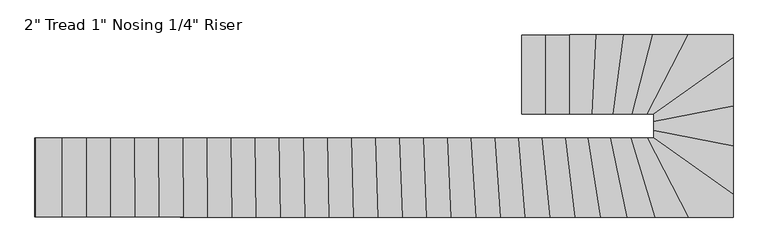
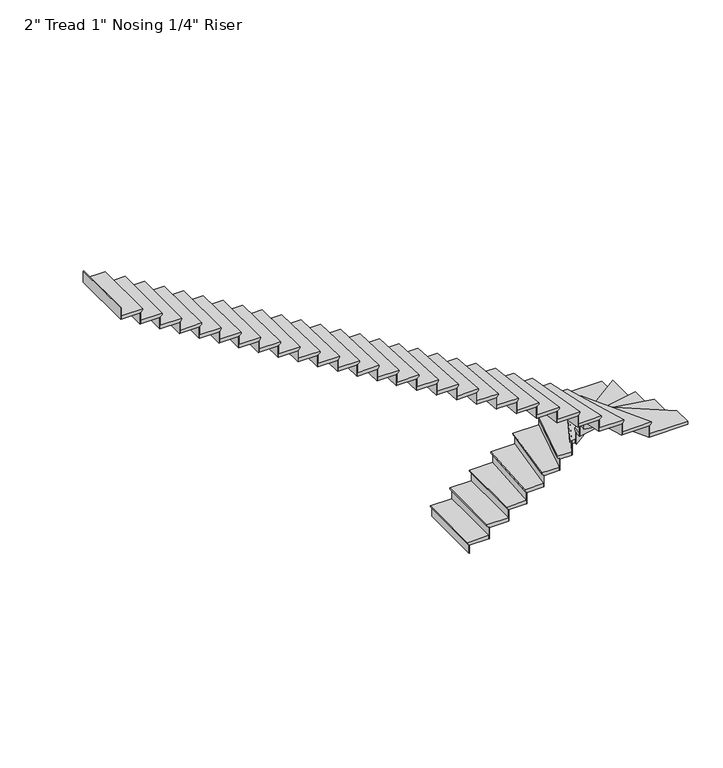
"""IFC4 building model written with IfcOpenShell, lengths in millimetres: stair flight geometry."""

from ifc_helpers import new_model, si_unit, origin, place, context, project, spatial, faceted_brep, source, transform, mapped, element, save


def stair_flight_225c1673(model_context):
    return source(origin(), model_context, "Body", "Brep", [
        faceted_brep([(11576.2992414, 57.0275916, 150.2833333), (11576.2992414, 57.0275916, 169.3333333), (11576.2992414, 971.4275916, 169.3333333), (11576.2992414, 971.4275916, 150.2833333), (11601.6992414, 57.0275916, 124.8833333), (11601.6992414, 971.4275916, 124.8833333), (11881.0992414, 57.0275916, 169.3333333), (11881.0992414, 971.4275916, 169.3333333), (11601.6992414, 971.4275916, 118.5333333), (11881.0992414, 971.4275916, 118.5333333), (11881.0992414, 57.0275916, 118.5333333), (11601.6992414, 57.0275916, 118.5333333)], [[[0, 1, 2, 3]], [[4, 0, 3, 5]], [[2, 1, 6, 7]], [[8, 9, 10, 11]], [[2, 7, 9, 8, 5, 3]], [[8, 11, 4, 5]], [[6, 1, 0, 4, 11, 10]], [[7, 6, 10, 9]]]),
        faceted_brep([(11601.6992414, 57.0275916, 118.5333333), (11601.6992414, 57.0275916, 0.0), (11608.0492414, 57.0275916, 0.0), (11608.0492414, 57.0275916, 118.5333333), (11601.6992414, 971.4275916, 118.5333333), (11608.0492414, 971.4275916, 118.5333333), (11608.0492414, 971.4275916, 0.0), (11601.6992414, 971.4275916, 0.0)], [[[0, 1, 2, 3]], [[4, 5, 6, 7]], [[1, 0, 4, 7]], [[2, 1, 7, 6]], [[3, 2, 6, 5]], [[0, 3, 5, 4]]]),
        faceted_brep([(11881.0992414, 57.0275916, 287.8666667), (11881.0992414, 57.0275916, 118.5333333), (11887.4492414, 57.0275916, 118.5333333), (11887.4492414, 57.0275916, 287.8666667), (11881.0992414, 971.4275916, 287.8666667), (11887.4492414, 971.4275916, 287.8666667), (11887.4492414, 971.4275916, 118.5333333), (11881.0992414, 971.4275916, 118.5333333)], [[[0, 1, 2, 3]], [[4, 5, 6, 7]], [[1, 0, 4, 7]], [[2, 1, 7, 6]], [[3, 2, 6, 5]], [[0, 3, 5, 4]]]),
        faceted_brep([(11855.6992414, 971.4275916, 338.6666667), (11855.6992414, 57.0275916, 338.6666667), (12160.4992414, 57.0275916, 338.6666667), (12160.4992414, 971.4275916, 338.6666667), (11881.0992414, 971.4275916, 287.8666667), (12160.4992414, 971.4275916, 287.8666667), (12160.4992414, 57.0275916, 287.8666667), (11881.0992414, 57.0275916, 287.8666667), (11881.0992414, 971.4275916, 294.2166667), (11855.6992414, 971.4275916, 319.6166667), (11881.0992414, 57.0275916, 294.2166667), (11855.6992414, 57.0275916, 319.6166667)], [[[0, 1, 2, 3]], [[4, 5, 6, 7]], [[0, 3, 5, 4, 8, 9]], [[4, 7, 10, 8]], [[2, 1, 11, 10, 7, 6]], [[3, 2, 6, 5]], [[11, 1, 0, 9]], [[10, 11, 9, 8]]]),
        faceted_brep([(12160.4992414, 57.0275916, 457.2), (12160.4992414, 57.0275916, 287.8666667), (12166.8492414, 57.0275916, 287.8666667), (12166.8492414, 57.0275916, 457.2), (12160.4992414, 971.4275916, 457.2), (12166.8492414, 971.4275916, 457.2), (12166.8492414, 971.4275916, 287.8666667), (12160.4992414, 971.4275916, 287.8666667)], [[[0, 1, 2, 3]], [[4, 5, 6, 7]], [[1, 0, 4, 7]], [[2, 1, 7, 6]], [[3, 2, 6, 5]], [[0, 3, 5, 4]]]),
        faceted_brep([(12135.0992414, 971.4275916, 508.0), (12135.0992414, 57.0275916, 508.0), (12416.1664028, 57.0275916, 508.0), (12463.7006732, 971.4275916, 508.0), (12160.4992414, 971.4275916, 457.2), (12463.7006732, 971.4275916, 457.2), (12416.1664028, 57.0275916, 457.2), (12160.4992414, 57.0275916, 457.2), (12160.4992414, 971.4275916, 463.55), (12135.0992414, 971.4275916, 488.95), (12160.4992414, 57.0275916, 463.55), (12135.0992414, 57.0275916, 488.95)], [[[0, 1, 2, 3]], [[4, 5, 6, 7]], [[0, 3, 5, 4, 8, 9]], [[4, 7, 10, 8]], [[2, 1, 11, 10, 7, 6]], [[3, 2, 6, 5]], [[11, 1, 0, 9]], [[10, 11, 9, 8]]]),
        faceted_brep([(12416.1664028, 57.0275916, 626.5333333), (12416.1664028, 57.0275916, 457.2), (12422.524977, 57.0275916, 457.2), (12422.524977, 57.0275916, 626.5333333), (12463.7006732, 971.4275916, 626.5333333), (12470.0592474, 971.4275916, 626.5333333), (12470.0592474, 971.4275916, 457.2), (12463.7006732, 971.4275916, 457.2)], [[[0, 1, 2, 3]], [[4, 5, 6, 7]], [[1, 0, 4, 7]], [[2, 1, 7, 6]], [[3, 2, 6, 5]], [[0, 3, 5, 4]]]),
        faceted_brep([(12438.2663766, 971.4275916, 677.3333333), (12390.7321062, 57.0275916, 677.3333333), (12660.3331027, 57.0275916, 677.3333333), (12778.6891543, 971.4275916, 677.3333333), (12463.7006732, 971.4275916, 626.5333333), (12778.6891543, 971.4275916, 626.5333333), (12660.3331027, 57.0275916, 626.5333333), (12416.1664028, 57.0275916, 626.5333333), (12463.7006732, 971.4275916, 632.8833333), (12438.2663766, 971.4275916, 658.2833333), (12416.1664028, 57.0275916, 632.8833333), (12390.7321062, 57.0275916, 658.2833333)], [[[0, 1, 2, 3]], [[4, 5, 6, 7]], [[0, 3, 5, 4, 8, 9]], [[4, 7, 10, 8]], [[2, 1, 11, 10, 7, 6]], [[3, 2, 6, 5]], [[11, 1, 0, 9]], [[10, 11, 9, 8]]]),
        faceted_brep([(12660.3331027, 57.0275916, 795.8666667), (12660.3331027, 57.0275916, 626.5333333), (12666.7360744, 57.0275916, 626.5333333), (12666.7360744, 57.0275916, 795.8666667), (12778.6891543, 971.4275916, 795.8666667), (12785.0921261, 971.4275916, 795.8666667), (12785.0921261, 971.4275916, 626.5333333), (12778.6891543, 971.4275916, 626.5333333)], [[[0, 1, 2, 3]], [[4, 5, 6, 7]], [[1, 0, 4, 7]], [[2, 1, 7, 6]], [[3, 2, 6, 5]], [[0, 3, 5, 4]]]),
        faceted_brep([(12753.0772672, 971.4275916, 846.6666667), (12634.7212156, 57.0275916, 846.6666667), (12881.9603251, 57.0275916, 846.6666667), (13117.0907726, 971.4275916, 846.6666667), (12778.6891543, 971.4275916, 795.8666667), (13117.0907726, 971.4275916, 795.8666667), (12881.9603251, 57.0275916, 795.8666667), (12660.3331027, 57.0275916, 795.8666667), (12778.6891543, 971.4275916, 802.2166667), (12753.0772672, 971.4275916, 827.6166667), (12660.3331027, 57.0275916, 802.2166667), (12634.7212156, 57.0275916, 827.6166667)], [[[0, 1, 2, 3]], [[4, 5, 6, 7]], [[0, 3, 5, 4, 8, 9]], [[4, 7, 10, 8]], [[2, 1, 11, 10, 7, 6]], [[3, 2, 6, 5]], [[11, 1, 0, 9]], [[10, 11, 9, 8]]]),
        faceted_brep([(12881.9603251, 57.0275916, 965.2), (12881.9603251, 57.0275916, 795.8666667), (12888.516902, 57.0275916, 795.8666667), (12888.516902, 57.0275916, 965.2), (13117.0907726, 971.4275916, 965.2), (13123.6473494, 971.4275916, 965.2), (13123.6473494, 971.4275916, 795.8666667), (13117.0907726, 971.4275916, 795.8666667)], [[[0, 1, 2, 3]], [[4, 5, 6, 7]], [[1, 0, 4, 7]], [[2, 1, 7, 6]], [[3, 2, 6, 5]], [[0, 3, 5, 4]]]),
        faceted_brep([(13090.8644651, 971.4275916, 1016.0), (12855.7340177, 57.0275916, 1016.0), (13058.3069612, 57.0275916, 1016.0), (13527.1315826, 971.4275916, 1016.0), (13117.0907726, 971.4275916, 965.2), (13527.1315826, 971.4275916, 965.2), (13058.3069612, 57.0275916, 965.2), (12881.9603251, 57.0275916, 965.2), (13117.0907726, 971.4275916, 971.55), (13090.8644651, 971.4275916, 996.95), (12881.9603251, 57.0275916, 971.55), (12855.7340177, 57.0275916, 996.95)], [[[0, 1, 2, 3]], [[4, 5, 6, 7]], [[0, 3, 5, 4, 8, 9]], [[4, 7, 10, 8]], [[2, 1, 11, 10, 7, 6]], [[3, 2, 6, 5]], [[11, 1, 0, 9]], [[10, 11, 9, 8]]]),
        faceted_brep([(13058.3069612, 57.0275916, 1134.5333333), (13058.3069612, 57.0275916, 965.2), (13065.4429444, 57.0275916, 965.2), (13065.4429444, 57.0275916, 1134.5333333), (13527.1315826, 971.4275916, 1134.5333333), (13534.2675657, 971.4275916, 1134.5333333), (13534.2675657, 971.4275916, 965.2), (13527.1315826, 971.4275916, 965.2)], [[[0, 1, 2, 3]], [[4, 5, 6, 7]], [[1, 0, 4, 7]], [[2, 1, 7, 6]], [[3, 2, 6, 5]], [[0, 3, 5, 4]]]),
        faceted_brep([(14018.4309332, 677.7464579, 1185.3333333), (14018.4309332, 971.4275916, 1185.3333333), (13498.58765, 971.4275916, 1185.3333333), (13029.7630287, 57.0275916, 1185.3333333), (13104.0309332, 57.0275916, 1185.3333333), (13104.0309332, 27.4725088, 1185.3333333), (14018.4309332, 971.4275916, 1134.5333333), (14018.4309332, 677.7464579, 1134.5333333), (13104.0309332, 27.4725088, 1134.5333333), (13104.0309332, 57.0275916, 1134.5333333), (13058.3069612, 57.0275916, 1134.5333333), (13527.1315826, 971.4275916, 1134.5333333), (13527.1315826, 971.4275916, 1140.8833333), (13498.58765, 971.4275916, 1166.2833333), (13058.3069612, 57.0275916, 1140.8833333), (13029.7630287, 57.0275916, 1166.2833333)], [[[0, 1, 2, 3, 4, 5]], [[6, 7, 8, 9, 10, 11]], [[1, 0, 7, 6]], [[2, 1, 6, 11, 12, 13]], [[11, 10, 14, 12]], [[4, 3, 15, 14, 10, 9]], [[5, 4, 9, 8]], [[0, 5, 8, 7]], [[15, 3, 2, 13]], [[14, 15, 13, 12]]]),
        faceted_brep([(13104.0309332, 27.4725088, 1303.8666667), (13104.0309332, 27.4725088, 1134.5333333), (13104.0309332, 19.680534, 1134.5333333), (13104.0309332, 19.680534, 1303.8666667), (14018.4309332, 677.7464579, 1303.8666667), (14018.4309332, 669.9544831, 1303.8666667), (14018.4309332, 669.9544831, 1134.5333333), (14018.4309332, 677.7464579, 1134.5333333)], [[[0, 1, 2, 3]], [[4, 5, 6, 7]], [[1, 0, 4, 7]], [[2, 1, 7, 6]], [[3, 2, 6, 5]], [[0, 3, 5, 4]]]),
        faceted_brep([(14018.4309332, 708.9143571, 1354.6666667), (13104.0309332, 58.6404079, 1354.6666667), (13104.0309332, -58.9815783, 1354.6666667), (14018.4309332, 121.259278, 1354.6666667), (14018.4309332, 677.7464579, 1303.8666667), (14018.4309332, 121.259278, 1303.8666667), (13104.0309332, -58.9815783, 1303.8666667), (13104.0309332, 27.4725088, 1303.8666667), (14018.4309332, 677.7464579, 1310.2166667), (14018.4309332, 708.9143571, 1335.6166667), (13104.0309332, 27.4725088, 1310.2166667), (13104.0309332, 58.6404079, 1335.6166667)], [[[0, 1, 2, 3]], [[4, 5, 6, 7]], [[0, 3, 5, 4, 8, 9]], [[4, 7, 10, 8]], [[2, 1, 11, 10, 7, 6]], [[3, 2, 6, 5]], [[11, 1, 0, 9]], [[10, 11, 9, 8]]]),
        faceted_brep([(13104.0309332, -58.9815783, 1473.2), (13104.0309332, -58.9815783, 1303.8666667), (13104.0309332, -65.4537637, 1303.8666667), (13104.0309332, -65.4537637, 1473.2), (14018.4309332, 121.259278, 1473.2), (14018.4309332, 114.7870926, 1473.2), (14018.4309332, 114.7870926, 1303.8666667), (14018.4309332, 121.259278, 1303.8666667)], [[[0, 1, 2, 3]], [[4, 5, 6, 7]], [[1, 0, 4, 7]], [[2, 1, 7, 6]], [[3, 2, 6, 5]], [[0, 3, 5, 4]]]),
        faceted_brep([(14018.4309332, 147.1480198, 1524.0), (13104.0309332, -33.0928366, 1524.0), (13104.0309332, -158.140722, 1524.0), (14018.4309332, -338.3815783, 1524.0), (14018.4309332, 121.259278, 1473.2), (14018.4309332, -338.3815783, 1473.2), (13104.0309332, -158.140722, 1473.2), (13104.0309332, -58.9815783, 1473.2), (14018.4309332, 121.259278, 1479.55), (14018.4309332, 147.1480198, 1504.95), (13104.0309332, -58.9815783, 1479.55), (13104.0309332, -33.0928366, 1504.95)], [[[0, 1, 2, 3]], [[4, 5, 6, 7]], [[0, 3, 5, 4, 8, 9]], [[4, 7, 10, 8]], [[2, 1, 11, 10, 7, 6]], [[3, 2, 6, 5]], [[11, 1, 0, 9]], [[10, 11, 9, 8]]]),
        faceted_brep([(13104.0309332, -158.140722, 1642.5333333), (13104.0309332, -158.140722, 1473.2), (13104.0309332, -164.6129074, 1473.2), (13104.0309332, -164.6129074, 1642.5333333), (14018.4309332, -338.3815783, 1642.5333333), (14018.4309332, -344.8537637, 1642.5333333), (14018.4309332, -344.8537637, 1473.2), (14018.4309332, -338.3815783, 1473.2)], [[[0, 1, 2, 3]], [[4, 5, 6, 7]], [[1, 0, 4, 7]], [[2, 1, 7, 6]], [[3, 2, 6, 5]], [[0, 3, 5, 4]]]),
        faceted_brep([(14018.4309332, -312.4928366, 1693.3333333), (13104.0309332, -132.2519802, 1693.3333333), (13104.0309332, -222.3724084, 1693.3333333), (13057.9354587, -222.3724084, 1693.3333333), (14018.4309332, -905.4270731, 1693.3333333), (14018.4309332, -338.3815783, 1642.5333333), (14018.4309332, -905.4270731, 1642.5333333), (13057.9354587, -222.3724084, 1642.5333333), (13104.0309332, -222.3724084, 1642.5333333), (13104.0309332, -158.140722, 1642.5333333), (14018.4309332, -338.3815783, 1648.8833333), (14018.4309332, -312.4928366, 1674.2833333), (13104.0309332, -158.140722, 1648.8833333), (13104.0309332, -132.2519802, 1674.2833333)], [[[0, 1, 2, 3, 4]], [[5, 6, 7, 8, 9]], [[0, 4, 6, 5, 10, 11]], [[5, 9, 12, 10]], [[2, 1, 13, 12, 9, 8]], [[3, 2, 8, 7]], [[4, 3, 7, 6]], [[13, 1, 0, 11]], [[12, 13, 11, 10]]]),
        faceted_brep([(13057.9354587, -222.3724084, 1811.8666667), (13057.9354587, -222.3724084, 1642.5333333), (13046.9785662, -222.3724084, 1642.5333333), (13046.9785662, -222.3724084, 1811.8666667), (14018.4309332, -905.4270731, 1811.8666667), (14018.4309332, -913.2190478, 1811.8666667), (14018.4309332, -913.2190478, 1642.5333333), (14018.4309332, -905.4270731, 1642.5333333)], [[[0, 1, 2, 3]], [[4, 5, 6, 7]], [[1, 0, 4, 7]], [[2, 1, 7, 6]], [[3, 2, 6, 5]], [[0, 3, 5, 4]]]),
        faceted_brep([(13470.0437175, -1136.7724084, 1862.6666667), (14018.4309332, -1136.7724084, 1862.6666667), (14018.4309332, -874.2591739, 1862.6666667), (13101.7630287, -222.3724084, 1862.6666667), (13001.2190962, -222.3724084, 1862.6666667), (14018.4309332, -1136.7724084, 1811.8666667), (13470.0437175, -1136.7724084, 1811.8666667), (13001.2190962, -222.3724084, 1811.8666667), (13057.9354587, -222.3724084, 1811.8666667), (14018.4309332, -905.4270731, 1811.8666667), (14018.4309332, -905.4270731, 1818.2166667), (14018.4309332, -874.2591739, 1843.6166667), (13057.9354587, -222.3724084, 1818.2166667), (13101.7630287, -222.3724084, 1843.6166667)], [[[0, 1, 2, 3, 4]], [[5, 6, 7, 8, 9]], [[1, 0, 6, 5]], [[2, 1, 5, 9, 10, 11]], [[9, 8, 12, 10]], [[4, 3, 13, 12, 8, 7]], [[0, 4, 7, 6]], [[13, 3, 2, 11]], [[12, 13, 11, 10]]]),
        faceted_brep([(13001.2190962, -222.3724084, 1981.2), (13001.2190962, -222.3724084, 1811.8666667), (12994.083113, -222.3724084, 1811.8666667), (12994.083113, -222.3724084, 1981.2), (13470.0437175, -1136.7724084, 1981.2), (13462.9077344, -1136.7724084, 1981.2), (13462.9077344, -1136.7724084, 1811.8666667), (13470.0437175, -1136.7724084, 1811.8666667)], [[[0, 1, 2, 3]], [[4, 5, 6, 7]], [[1, 0, 4, 7]], [[2, 1, 7, 6]], [[3, 2, 6, 5]], [[0, 3, 5, 4]]]),
        faceted_brep([(13498.58765, -1136.7724084, 2032.0), (13029.7630287, -222.3724084, 2032.0), (12807.3925391, -222.3724084, 2032.0), (13086.0986548, -1136.7724084, 2032.0), (13470.0437175, -1136.7724084, 1981.2), (13086.0986548, -1136.7724084, 1981.2), (12807.3925391, -222.3724084, 1981.2), (13001.2190962, -222.3724084, 1981.2), (13470.0437175, -1136.7724084, 1987.55), (13498.58765, -1136.7724084, 2012.95), (13001.2190962, -222.3724084, 1987.55), (13029.7630287, -222.3724084, 2012.95)], [[[0, 1, 2, 3]], [[4, 5, 6, 7]], [[0, 3, 5, 4, 8, 9]], [[4, 7, 10, 8]], [[2, 1, 11, 10, 7, 6]], [[3, 2, 6, 5]], [[11, 1, 0, 9]], [[10, 11, 9, 8]]]),
        faceted_brep([(12807.3925391, -222.3724084, 2150.5333333), (12807.3925391, -222.3724084, 1981.2), (12800.754128, -222.3724084, 1981.2), (12800.754128, -222.3724084, 2150.5333333), (13086.0986548, -1136.7724084, 2150.5333333), (13079.4602437, -1136.7724084, 2150.5333333), (13079.4602437, -1136.7724084, 1981.2), (13086.0986548, -1136.7724084, 1981.2)], [[[0, 1, 2, 3]], [[4, 5, 6, 7]], [[1, 0, 4, 7]], [[2, 1, 7, 6]], [[3, 2, 6, 5]], [[0, 3, 5, 4]]]),
        faceted_brep([(13112.6522993, -1136.7724084, 2201.3333333), (12833.9461835, -222.3724084, 2201.3333333), (12571.2502843, -222.3724084, 2201.3333333), (12764.6246729, -1136.7724084, 2201.3333333), (13086.0986548, -1136.7724084, 2150.5333333), (12764.6246729, -1136.7724084, 2150.5333333), (12571.2502843, -222.3724084, 2150.5333333), (12807.3925391, -222.3724084, 2150.5333333), (13086.0986548, -1136.7724084, 2156.8833333), (13112.6522993, -1136.7724084, 2182.2833333), (12807.3925391, -222.3724084, 2156.8833333), (12833.9461835, -222.3724084, 2182.2833333)], [[[0, 1, 2, 3]], [[4, 5, 6, 7]], [[0, 3, 5, 4, 8, 9]], [[4, 7, 10, 8]], [[2, 1, 11, 10, 7, 6]], [[3, 2, 6, 5]], [[11, 1, 0, 9]], [[10, 11, 9, 8]]]),
        faceted_brep([(12571.2502843, -222.3724084, 2319.8666667), (12571.2502843, -222.3724084, 2150.5333333), (12564.7598436, -222.3724084, 2150.5333333), (12564.7598436, -222.3724084, 2319.8666667), (12764.6246729, -1136.7724084, 2319.8666667), (12758.1342322, -1136.7724084, 2319.8666667), (12758.1342322, -1136.7724084, 2150.5333333), (12764.6246729, -1136.7724084, 2150.5333333)], [[[0, 1, 2, 3]], [[4, 5, 6, 7]], [[1, 0, 4, 7]], [[2, 1, 7, 6]], [[3, 2, 6, 5]], [[0, 3, 5, 4]]]),
        faceted_brep([(12790.5864357, -1136.7724084, 2370.6666667), (12597.2120471, -222.3724084, 2370.6666667), (12316.3757237, -222.3724084, 2370.6666667), (12461.1896421, -1136.7724084, 2370.6666667), (12764.6246729, -1136.7724084, 2319.8666667), (12461.1896421, -1136.7724084, 2319.8666667), (12316.3757237, -222.3724084, 2319.8666667), (12571.2502843, -222.3724084, 2319.8666667), (12764.6246729, -1136.7724084, 2326.2166667), (12790.5864357, -1136.7724084, 2351.6166667), (12571.2502843, -222.3724084, 2326.2166667), (12597.2120471, -222.3724084, 2351.6166667)], [[[0, 1, 2, 3]], [[4, 5, 6, 7]], [[0, 3, 5, 4, 8, 9]], [[4, 7, 10, 8]], [[2, 1, 11, 10, 7, 6]], [[3, 2, 6, 5]], [[11, 1, 0, 9]], [[10, 11, 9, 8]]]),
        faceted_brep([(12316.3757237, -222.3724084, 2489.2), (12316.3757237, -222.3724084, 2319.8666667), (12309.946584, -222.3724084, 2319.8666667), (12309.946584, -222.3724084, 2489.2), (12461.1896421, -1136.7724084, 2489.2), (12454.7605024, -1136.7724084, 2489.2), (12454.7605024, -1136.7724084, 2319.8666667), (12461.1896421, -1136.7724084, 2319.8666667)], [[[0, 1, 2, 3]], [[4, 5, 6, 7]], [[1, 0, 4, 7]], [[2, 1, 7, 6]], [[3, 2, 6, 5]], [[0, 3, 5, 4]]]),
        faceted_brep([(12486.9062006, -1136.7724084, 2540.0), (12342.0922822, -222.3724084, 2540.0), (12052.7695473, -222.3724084, 2540.0), (12166.2392994, -1136.7724084, 2540.0), (12461.1896421, -1136.7724084, 2489.2), (12166.2392994, -1136.7724084, 2489.2), (12052.7695473, -222.3724084, 2489.2), (12316.3757237, -222.3724084, 2489.2), (12461.1896421, -1136.7724084, 2495.55), (12486.9062006, -1136.7724084, 2520.95), (12316.3757237, -222.3724084, 2495.55), (12342.0922822, -222.3724084, 2520.95)], [[[0, 1, 2, 3]], [[4, 5, 6, 7]], [[0, 3, 5, 4, 8, 9]], [[4, 7, 10, 8]], [[2, 1, 11, 10, 7, 6]], [[3, 2, 6, 5]], [[11, 1, 0, 9]], [[10, 11, 9, 8]]]),
        faceted_brep([(12052.7695473, -222.3724084, 2658.5333333), (12052.7695473, -222.3724084, 2489.2), (12046.3708427, -222.3724084, 2489.2), (12046.3708427, -222.3724084, 2658.5333333), (12166.2392994, -1136.7724084, 2658.5333333), (12159.8405949, -1136.7724084, 2658.5333333), (12159.8405949, -1136.7724084, 2489.2), (12166.2392994, -1136.7724084, 2489.2)], [[[0, 1, 2, 3]], [[4, 5, 6, 7]], [[1, 0, 4, 7]], [[2, 1, 7, 6]], [[3, 2, 6, 5]], [[0, 3, 5, 4]]]),
        faceted_brep([(12191.8341175, -1136.7724084, 2709.3333333), (12078.3643653, -222.3724084, 2709.3333333), (11784.3897784, -222.3724084, 2709.3333333), (11875.9546455, -1136.7724084, 2709.3333333), (12166.2392994, -1136.7724084, 2658.5333333), (11875.9546455, -1136.7724084, 2658.5333333), (11784.3897784, -222.3724084, 2658.5333333), (12052.7695473, -222.3724084, 2658.5333333), (12166.2392994, -1136.7724084, 2664.8833333), (12191.8341175, -1136.7724084, 2690.2833333), (12052.7695473, -222.3724084, 2664.8833333), (12078.3643653, -222.3724084, 2690.2833333)], [[[0, 1, 2, 3]], [[4, 5, 6, 7]], [[0, 3, 5, 4, 8, 9]], [[4, 7, 10, 8]], [[2, 1, 11, 10, 7, 6]], [[3, 2, 6, 5]], [[11, 1, 0, 9]], [[10, 11, 9, 8]]]),
        faceted_brep([(11784.3897784, -222.3724084, 2827.8666667), (11784.3897784, -222.3724084, 2658.5333333), (11778.008021, -222.3724084, 2658.5333333), (11778.008021, -222.3724084, 2827.8666667), (11875.9546455, -1136.7724084, 2827.8666667), (11869.5728881, -1136.7724084, 2827.8666667), (11869.5728881, -1136.7724084, 2658.5333333), (11875.9546455, -1136.7724084, 2658.5333333)], [[[0, 1, 2, 3]], [[4, 5, 6, 7]], [[1, 0, 4, 7]], [[2, 1, 7, 6]], [[3, 2, 6, 5]], [[0, 3, 5, 4]]]),
        faceted_brep([(11901.4816749, -1136.7724084, 2878.6666667), (11809.9168078, -222.3724084, 2878.6666667), (11513.1163854, -222.3724084, 2878.6666667), (11588.5097158, -1136.7724084, 2878.6666667), (11875.9546455, -1136.7724084, 2827.8666667), (11588.5097158, -1136.7724084, 2827.8666667), (11513.1163854, -222.3724084, 2827.8666667), (11784.3897784, -222.3724084, 2827.8666667), (11875.9546455, -1136.7724084, 2834.2166667), (11901.4816749, -1136.7724084, 2859.6166667), (11784.3897784, -222.3724084, 2834.2166667), (11809.9168078, -222.3724084, 2859.6166667)], [[[0, 1, 2, 3]], [[4, 5, 6, 7]], [[0, 3, 5, 4, 8, 9]], [[4, 7, 10, 8]], [[2, 1, 11, 10, 7, 6]], [[3, 2, 6, 5]], [[11, 1, 0, 9]], [[10, 11, 9, 8]]]),
        faceted_brep([(11513.1163854, -222.3724084, 2997.2), (11513.1163854, -222.3724084, 2827.8666667), (11506.7448377, -222.3724084, 2827.8666667), (11506.7448377, -222.3724084, 2997.2), (11588.5097158, -1136.7724084, 2997.2), (11582.1381681, -1136.7724084, 2997.2), (11582.1381681, -1136.7724084, 2827.8666667), (11588.5097158, -1136.7724084, 2827.8666667)], [[[0, 1, 2, 3]], [[4, 5, 6, 7]], [[1, 0, 4, 7]], [[2, 1, 7, 6]], [[3, 2, 6, 5]], [[0, 3, 5, 4]]]),
        faceted_brep([(11613.9959066, -1136.7724084, 3048.0), (11538.6025762, -222.3724084, 3048.0), (11239.9567563, -222.3724084, 3048.0), (11302.9214332, -1136.7724084, 3048.0), (11588.5097158, -1136.7724084, 2997.2), (11302.9214332, -1136.7724084, 2997.2), (11239.9567563, -222.3724084, 2997.2), (11513.1163854, -222.3724084, 2997.2), (11588.5097158, -1136.7724084, 3003.55), (11613.9959066, -1136.7724084, 3028.95), (11513.1163854, -222.3724084, 3003.55), (11538.6025762, -222.3724084, 3028.95)], [[[0, 1, 2, 3]], [[4, 5, 6, 7]], [[0, 3, 5, 4, 8, 9]], [[4, 7, 10, 8]], [[2, 1, 11, 10, 7, 6]], [[3, 2, 6, 5]], [[11, 1, 0, 9]], [[10, 11, 9, 8]]]),
        faceted_brep([(11239.9567563, -222.3724084, 3166.5333333), (11239.9567563, -222.3724084, 2997.2), (11233.5917197, -222.3724084, 2997.2), (11233.5917197, -222.3724084, 3166.5333333), (11302.9214332, -1136.7724084, 3166.5333333), (11296.5563965, -1136.7724084, 3166.5333333), (11296.5563965, -1136.7724084, 2997.2), (11302.9214332, -1136.7724084, 2997.2)], [[[0, 1, 2, 3]], [[4, 5, 6, 7]], [[1, 0, 4, 7]], [[2, 1, 7, 6]], [[3, 2, 6, 5]], [[0, 3, 5, 4]]]),
        faceted_brep([(11328.3815798, -1136.7724084, 3217.3333333), (11265.416903, -222.3724084, 3217.3333333), (10965.4992991, -222.3724084, 3217.3333333), (11018.6135553, -1136.7724084, 3217.3333333), (11302.9214332, -1136.7724084, 3166.5333333), (11018.6135553, -1136.7724084, 3166.5333333), (10965.4992991, -222.3724084, 3166.5333333), (11239.9567563, -222.3724084, 3166.5333333), (11302.9214332, -1136.7724084, 3172.8833333), (11328.3815798, -1136.7724084, 3198.2833333), (11239.9567563, -222.3724084, 3172.8833333), (11265.416903, -222.3724084, 3198.2833333)], [[[0, 1, 2, 3]], [[4, 5, 6, 7]], [[0, 3, 5, 4, 8, 9]], [[4, 7, 10, 8]], [[2, 1, 11, 10, 7, 6]], [[3, 2, 6, 5]], [[11, 1, 0, 9]], [[10, 11, 9, 8]]]),
        faceted_brep([(10965.4992991, -222.3724084, 3335.8666667), (10965.4992991, -222.3724084, 3166.5333333), (10959.1385956, -222.3724084, 3166.5333333), (10959.1385956, -222.3724084, 3335.8666667), (11018.6135553, -1136.7724084, 3335.8666667), (11012.2528517, -1136.7724084, 3335.8666667), (11012.2528517, -1136.7724084, 3166.5333333), (11018.6135553, -1136.7724084, 3166.5333333)], [[[0, 1, 2, 3]], [[4, 5, 6, 7]], [[1, 0, 4, 7]], [[2, 1, 7, 6]], [[3, 2, 6, 5]], [[0, 3, 5, 4]]]),
        faceted_brep([(11044.0563695, -1136.7724084, 3386.6666667), (10990.9421133, -222.3724084, 3386.6666667), (10690.1107415, -222.3724084, 3386.6666667), (10735.2259477, -1136.7724084, 3386.6666667), (11018.6135553, -1136.7724084, 3335.8666667), (10735.2259477, -1136.7724084, 3335.8666667), (10690.1107415, -222.3724084, 3335.8666667), (10965.4992991, -222.3724084, 3335.8666667), (11018.6135553, -1136.7724084, 3342.2166667), (11044.0563695, -1136.7724084, 3367.6166667), (10965.4992991, -222.3724084, 3342.2166667), (10990.9421133, -222.3724084, 3367.6166667)], [[[0, 1, 2, 3]], [[4, 5, 6, 7]], [[0, 3, 5, 4, 8, 9]], [[4, 7, 10, 8]], [[2, 1, 11, 10, 7, 6]], [[3, 2, 6, 5]], [[11, 1, 0, 9]], [[10, 11, 9, 8]]]),
        faceted_brep([(10690.1107415, -222.3724084, 3505.2), (10690.1107415, -222.3724084, 3335.8666667), (10683.7530173, -222.3724084, 3335.8666667), (10683.7530173, -222.3724084, 3505.2), (10735.2259477, -1136.7724084, 3505.2), (10728.8682235, -1136.7724084, 3505.2), (10728.8682235, -1136.7724084, 3335.8666667), (10735.2259477, -1136.7724084, 3335.8666667)], [[[0, 1, 2, 3]], [[4, 5, 6, 7]], [[1, 0, 4, 7]], [[2, 1, 7, 6]], [[3, 2, 6, 5]], [[0, 3, 5, 4]]]),
        faceted_brep([(10760.6568445, -1136.7724084, 3556.0), (10715.5416383, -222.3724084, 3556.0), (10414.0315388, -222.3724084, 3556.0), (10452.5219583, -1136.7724084, 3556.0), (10735.2259477, -1136.7724084, 3505.2), (10452.5219583, -1136.7724084, 3505.2), (10414.0315388, -222.3724084, 3505.2), (10690.1107415, -222.3724084, 3505.2), (10735.2259477, -1136.7724084, 3511.55), (10760.6568445, -1136.7724084, 3536.95), (10690.1107415, -222.3724084, 3511.55), (10715.5416383, -222.3724084, 3536.95)], [[[0, 1, 2, 3]], [[4, 5, 6, 7]], [[0, 3, 5, 4, 8, 9]], [[4, 7, 10, 8]], [[2, 1, 11, 10, 7, 6]], [[3, 2, 6, 5]], [[11, 1, 0, 9]], [[10, 11, 9, 8]]]),
        faceted_brep([(10414.0315388, -222.3724084, 3674.5333333), (10414.0315388, -222.3724084, 3505.2), (10407.6759156, -222.3724084, 3505.2), (10407.6759156, -222.3724084, 3674.5333333), (10452.5219583, -1136.7724084, 3674.5333333), (10446.1663351, -1136.7724084, 3674.5333333), (10446.1663351, -1136.7724084, 3505.2), (10452.5219583, -1136.7724084, 3505.2)], [[[0, 1, 2, 3]], [[4, 5, 6, 7]], [[1, 0, 4, 7]], [[2, 1, 7, 6]], [[3, 2, 6, 5]], [[0, 3, 5, 4]]]),
        faceted_brep([(10477.9444511, -1136.7724084, 3725.3333333), (10439.4540316, -222.3724084, 3725.3333333), (10137.4259134, -222.3724084, 3725.3333333), (10170.3396709, -1136.7724084, 3725.3333333), (10452.5219583, -1136.7724084, 3674.5333333), (10170.3396709, -1136.7724084, 3674.5333333), (10137.4259134, -222.3724084, 3674.5333333), (10414.0315388, -222.3724084, 3674.5333333), (10452.5219583, -1136.7724084, 3680.8833333), (10477.9444511, -1136.7724084, 3706.2833333), (10414.0315388, -222.3724084, 3680.8833333), (10439.4540316, -222.3724084, 3706.2833333)], [[[0, 1, 2, 3]], [[4, 5, 6, 7]], [[0, 3, 5, 4, 8, 9]], [[4, 7, 10, 8]], [[2, 1, 11, 10, 7, 6]], [[3, 2, 6, 5]], [[11, 1, 0, 9]], [[10, 11, 9, 8]]]),
        faceted_brep([(10137.4259134, -222.3724084, 3843.8666667), (10137.4259134, -222.3724084, 3674.5333333), (10131.0718011, -222.3724084, 3674.5333333), (10131.0718011, -222.3724084, 3843.8666667), (10170.3396709, -1136.7724084, 3843.8666667), (10163.9855586, -1136.7724084, 3843.8666667), (10163.9855586, -1136.7724084, 3674.5333333), (10170.3396709, -1136.7724084, 3674.5333333)], [[[0, 1, 2, 3]], [[4, 5, 6, 7]], [[1, 0, 4, 7]], [[2, 1, 7, 6]], [[3, 2, 6, 5]], [[0, 3, 5, 4]]]),
        faceted_brep([(10195.7561201, -1136.7724084, 3894.6666667), (10162.8423626, -222.3724084, 3894.6666667), (9860.4098466, -222.3724084, 3894.6666667), (9888.5645615, -1136.7724084, 3894.6666667), (10170.3396709, -1136.7724084, 3843.8666667), (9888.5645615, -1136.7724084, 3843.8666667), (9860.4098466, -222.3724084, 3843.8666667), (10137.4259134, -222.3724084, 3843.8666667), (10170.3396709, -1136.7724084, 3850.2166667), (10195.7561201, -1136.7724084, 3875.6166667), (10137.4259134, -222.3724084, 3850.2166667), (10162.8423626, -222.3724084, 3875.6166667)], [[[0, 1, 2, 3]], [[4, 5, 6, 7]], [[0, 3, 5, 4, 8, 9]], [[4, 7, 10, 8]], [[2, 1, 11, 10, 7, 6]], [[3, 2, 6, 5]], [[11, 1, 0, 9]], [[10, 11, 9, 8]]]),
        faceted_brep([(9860.4098466, -222.3724084, 4013.2), (9860.4098466, -222.3724084, 3843.8666667), (9854.0568373, -222.3724084, 3843.8666667), (9854.0568373, -222.3724084, 4013.2), (9888.5645615, -1136.7724084, 4013.2), (9882.2115521, -1136.7724084, 4013.2), (9882.2115521, -1136.7724084, 3843.8666667), (9888.5645615, -1136.7724084, 3843.8666667)], [[[0, 1, 2, 3]], [[4, 5, 6, 7]], [[1, 0, 4, 7]], [[2, 1, 7, 6]], [[3, 2, 6, 5]], [[0, 3, 5, 4]]]),
        faceted_brep([(9913.9765988, -1136.7724084, 4064.0), (9885.821884, -222.3724084, 4064.0), (9583.0675804, -222.3724084, 4064.0), (9607.1133408, -1136.7724084, 4064.0), (9888.5645615, -1136.7724084, 4013.2), (9607.1133408, -1136.7724084, 4013.2), (9583.0675804, -222.3724084, 4013.2), (9860.4098466, -222.3724084, 4013.2), (9888.5645615, -1136.7724084, 4019.55), (9913.9765988, -1136.7724084, 4044.95), (9860.4098466, -222.3724084, 4019.55), (9885.821884, -222.3724084, 4044.95)], [[[0, 1, 2, 3]], [[4, 5, 6, 7]], [[0, 3, 5, 4, 8, 9]], [[4, 7, 10, 8]], [[2, 1, 11, 10, 7, 6]], [[3, 2, 6, 5]], [[11, 1, 0, 9]], [[10, 11, 9, 8]]]),
        faceted_brep([(9583.0675804, -222.3724084, 4182.5333333), (9583.0675804, -222.3724084, 4013.2), (9576.7153852, -222.3724084, 4013.2), (9576.7153852, -222.3724084, 4182.5333333), (9607.1133408, -1136.7724084, 4182.5333333), (9600.7611456, -1136.7724084, 4182.5333333), (9600.7611456, -1136.7724084, 4013.2), (9607.1133408, -1136.7724084, 4013.2)], [[[0, 1, 2, 3]], [[4, 5, 6, 7]], [[1, 0, 4, 7]], [[2, 1, 7, 6]], [[3, 2, 6, 5]], [[0, 3, 5, 4]]]),
        faceted_brep([(9632.5221216, -1136.7724084, 4233.3333333), (9608.4763612, -222.3724084, 4233.3333333), (9305.461779, -222.3724084, 4233.3333333), (9325.9239859, -1136.7724084, 4233.3333333), (9607.1133408, -1136.7724084, 4182.5333333), (9325.9239859, -1136.7724084, 4182.5333333), (9305.461779, -222.3724084, 4182.5333333), (9583.0675804, -222.3724084, 4182.5333333), (9607.1133408, -1136.7724084, 4188.8833333), (9632.5221216, -1136.7724084, 4214.2833333), (9583.0675804, -222.3724084, 4188.8833333), (9608.4763612, -222.3724084, 4214.2833333)], [[[0, 1, 2, 3]], [[4, 5, 6, 7]], [[0, 3, 5, 4, 8, 9]], [[4, 7, 10, 8]], [[2, 1, 11, 10, 7, 6]], [[3, 2, 6, 5]], [[11, 1, 0, 9]], [[10, 11, 9, 8]]]),
        faceted_brep([(9305.461779, -222.3724084, 4351.8666667), (9305.461779, -222.3724084, 4182.5333333), (9299.1101893, -222.3724084, 4182.5333333), (9299.1101893, -222.3724084, 4351.8666667), (9325.9239859, -1136.7724084, 4351.8666667), (9319.5723962, -1136.7724084, 4351.8666667), (9319.5723962, -1136.7724084, 4182.5333333), (9325.9239859, -1136.7724084, 4182.5333333)], [[[0, 1, 2, 3]], [[4, 5, 6, 7]], [[1, 0, 4, 7]], [[2, 1, 7, 6]], [[3, 2, 6, 5]], [[0, 3, 5, 4]]]),
        faceted_brep([(9351.3303448, -1136.7724084, 4402.6666667), (9330.8681379, -222.3724084, 4402.6666667), (9027.6400223, -222.3724084, 4402.6666667), (9044.9493596, -1136.7724084, 4402.6666667), (9325.9239859, -1136.7724084, 4351.8666667), (9044.9493596, -1136.7724084, 4351.8666667), (9027.6400223, -222.3724084, 4351.8666667), (9305.461779, -222.3724084, 4351.8666667), (9325.9239859, -1136.7724084, 4358.2166667), (9351.3303448, -1136.7724084, 4383.6166667), (9305.461779, -222.3724084, 4358.2166667), (9330.8681379, -222.3724084, 4383.6166667)], [[[0, 1, 2, 3]], [[4, 5, 6, 7]], [[0, 3, 5, 4, 8, 9]], [[4, 7, 10, 8]], [[2, 1, 11, 10, 7, 6]], [[3, 2, 6, 5]], [[11, 1, 0, 9]], [[10, 11, 9, 8]]]),
        faceted_brep([(9027.6400223, -222.3724084, 4521.2), (9027.6400223, -222.3724084, 4351.8666667), (9021.2888847, -222.3724084, 4351.8666667), (9021.2888847, -222.3724084, 4521.2), (9044.9493596, -1136.7724084, 4521.2), (9038.598222, -1136.7724084, 4521.2), (9038.598222, -1136.7724084, 4351.8666667), (9044.9493596, -1136.7724084, 4351.8666667)], [[[0, 1, 2, 3]], [[4, 5, 6, 7]], [[1, 0, 4, 7]], [[2, 1, 7, 6]], [[3, 2, 6, 5]], [[0, 3, 5, 4]]]),
        faceted_brep([(9070.35391, -1136.7724084, 4572.0), (9053.0445727, -222.3724084, 4572.0), (8749.6390863, -222.3724084, 4572.0), (8764.1529976, -1136.7724084, 4572.0), (9044.9493596, -1136.7724084, 4521.2), (8764.1529976, -1136.7724084, 4521.2), (8749.6390863, -222.3724084, 4521.2), (9027.6400223, -222.3724084, 4521.2), (9044.9493596, -1136.7724084, 4527.55), (9070.35391, -1136.7724084, 4552.95), (9027.6400223, -222.3724084, 4527.55), (9053.0445727, -222.3724084, 4552.95)], [[[0, 1, 2, 3]], [[4, 5, 6, 7]], [[0, 3, 5, 4, 8, 9]], [[4, 7, 10, 8]], [[2, 1, 11, 10, 7, 6]], [[3, 2, 6, 5]], [[11, 1, 0, 9]], [[10, 11, 9, 8]]]),
        faceted_brep([(8749.6390863, -222.3724084, 4690.5333333), (8749.6390863, -222.3724084, 4521.2), (8743.2882865, -222.3724084, 4521.2), (8743.2882865, -222.3724084, 4690.5333333), (8764.1529976, -1136.7724084, 4690.5333333), (8757.8021977, -1136.7724084, 4690.5333333), (8757.8021977, -1136.7724084, 4521.2), (8764.1529976, -1136.7724084, 4521.2)], [[[0, 1, 2, 3]], [[4, 5, 6, 7]], [[1, 0, 4, 7]], [[2, 1, 7, 6]], [[3, 2, 6, 5]], [[0, 3, 5, 4]]]),
        faceted_brep([(8789.556197, -1136.7724084, 4741.3333333), (8775.0422858, -222.3724084, 4741.3333333), (8471.4878455, -222.3724084, 4741.3333333), (8483.5062495, -1136.7724084, 4741.3333333), (8764.1529976, -1136.7724084, 4690.5333333), (8483.5062495, -1136.7724084, 4690.5333333), (8471.4878455, -222.3724084, 4690.5333333), (8749.6390863, -222.3724084, 4690.5333333), (8764.1529976, -1136.7724084, 4696.8833333), (8789.556197, -1136.7724084, 4722.2833333), (8749.6390863, -222.3724084, 4696.8833333), (8775.0422858, -222.3724084, 4722.2833333)], [[[0, 1, 2, 3]], [[4, 5, 6, 7]], [[0, 3, 5, 4, 8, 9]], [[4, 7, 10, 8]], [[2, 1, 11, 10, 7, 6]], [[3, 2, 6, 5]], [[11, 1, 0, 9]], [[10, 11, 9, 8]]]),
        faceted_brep([(8471.4878455, -222.3724084, 4859.8666667), (8471.4878455, -222.3724084, 4690.5333333), (8465.1372971, -222.3724084, 4690.5333333), (8465.1372971, -222.3724084, 4859.8666667), (8483.5062495, -1136.7724084, 4859.8666667), (8477.1557011, -1136.7724084, 4859.8666667), (8477.1557011, -1136.7724084, 4690.5333333), (8483.5062495, -1136.7724084, 4690.5333333)], [[[0, 1, 2, 3]], [[4, 5, 6, 7]], [[1, 0, 4, 7]], [[2, 1, 7, 6]], [[3, 2, 6, 5]], [[0, 3, 5, 4]]]),
        faceted_brep([(8508.9084434, -1136.7724084, 4910.6666667), (8496.8900394, -222.3724084, 4910.6666667), (8193.2092865, -222.3724084, 4910.6666667), (8202.9862925, -1136.7724084, 4910.6666667), (8483.5062495, -1136.7724084, 4859.8666667), (8202.9862925, -1136.7724084, 4859.8666667), (8193.2092865, -222.3724084, 4859.8666667), (8471.4878455, -222.3724084, 4859.8666667), (8483.5062495, -1136.7724084, 4866.2166667), (8508.9084434, -1136.7724084, 4891.6166667), (8471.4878455, -222.3724084, 4866.2166667), (8496.8900394, -222.3724084, 4891.6166667)], [[[0, 1, 2, 3]], [[4, 5, 6, 7]], [[0, 3, 5, 4, 8, 9]], [[4, 7, 10, 8]], [[2, 1, 11, 10, 7, 6]], [[3, 2, 6, 5]], [[11, 1, 0, 9]], [[10, 11, 9, 8]]]),
        faceted_brep([(8193.2092865, -222.3724084, 5029.2), (8193.2092865, -222.3724084, 4859.8666667), (8186.8589236, -222.3724084, 4859.8666667), (8186.8589236, -222.3724084, 5029.2), (8202.9862925, -1136.7724084, 5029.2), (8196.6359295, -1136.7724084, 5029.2), (8196.6359295, -1136.7724084, 4859.8666667), (8202.9862925, -1136.7724084, 4859.8666667)], [[[0, 1, 2, 3]], [[4, 5, 6, 7]], [[1, 0, 4, 7]], [[2, 1, 7, 6]], [[3, 2, 6, 5]], [[0, 3, 5, 4]]]),
        faceted_brep([(8228.3877444, -1136.7724084, 5080.0), (8218.6107384, -222.3724084, 5080.0), (7914.821936, -222.3724084, 5080.0), (7922.5747209, -1136.7724084, 5080.0), (8202.9862925, -1136.7724084, 5029.2), (7922.5747209, -1136.7724084, 5029.2), (7914.821936, -222.3724084, 5029.2), (8193.2092865, -222.3724084, 5029.2), (8202.9862925, -1136.7724084, 5035.55), (8228.3877444, -1136.7724084, 5060.95), (8193.2092865, -222.3724084, 5035.55), (8218.6107384, -222.3724084, 5060.95)], [[[0, 1, 2, 3]], [[4, 5, 6, 7]], [[0, 3, 5, 4, 8, 9]], [[4, 7, 10, 8]], [[2, 1, 11, 10, 7, 6]], [[3, 2, 6, 5]], [[11, 1, 0, 9]], [[10, 11, 9, 8]]]),
        faceted_brep([(7914.821936, -222.3724084, 5198.5333333), (7914.821936, -222.3724084, 5029.2), (7908.4717078, -222.3724084, 5029.2), (7908.4717078, -222.3724084, 5198.5333333), (7922.5747209, -1136.7724084, 5198.5333333), (7916.2244926, -1136.7724084, 5198.5333333), (7916.2244926, -1136.7724084, 5029.2), (7922.5747209, -1136.7724084, 5029.2)], [[[0, 1, 2, 3]], [[4, 5, 6, 7]], [[1, 0, 4, 7]], [[2, 1, 7, 6]], [[3, 2, 6, 5]], [[0, 3, 5, 4]]]),
        faceted_brep([(7947.9756338, -1136.7724084, 5249.3333333), (7940.222849, -222.3724084, 5249.3333333), (7636.3408926, -222.3724084, 5249.3333333), (7642.2565271, -1136.7724084, 5249.3333333), (7922.5747209, -1136.7724084, 5198.5333333), (7642.2565271, -1136.7724084, 5198.5333333), (7636.3408926, -222.3724084, 5198.5333333), (7914.821936, -222.3724084, 5198.5333333), (7922.5747209, -1136.7724084, 5204.8833333), (7947.9756338, -1136.7724084, 5230.2833333), (7914.821936, -222.3724084, 5204.8833333), (7940.222849, -222.3724084, 5230.2833333)], [[[0, 1, 2, 3]], [[4, 5, 6, 7]], [[0, 3, 5, 4, 8, 9]], [[4, 7, 10, 8]], [[2, 1, 11, 10, 7, 6]], [[3, 2, 6, 5]], [[11, 1, 0, 9]], [[10, 11, 9, 8]]]),
        faceted_brep([(7636.3408926, -222.3724084, 5367.8666667), (7636.3408926, -222.3724084, 5198.5333333), (7629.9907597, -222.3724084, 5198.5333333), (7629.9907597, -222.3724084, 5367.8666667), (7642.2565271, -1136.7724084, 5367.8666667), (7635.9063943, -1136.7724084, 5367.8666667), (7635.9063943, -1136.7724084, 5198.5333333), (7642.2565271, -1136.7724084, 5198.5333333)], [[[0, 1, 2, 3]], [[4, 5, 6, 7]], [[1, 0, 4, 7]], [[2, 1, 7, 6]], [[3, 2, 6, 5]], [[0, 3, 5, 4]]]),
        faceted_brep([(7667.6570587, -1136.7724084, 5418.6666667), (7661.7414241, -222.3724084, 5418.6666667), (7357.7785842, -222.3724084, 5418.6666667), (7362.0193522, -1136.7724084, 5418.6666667), (7642.2565271, -1136.7724084, 5367.8666667), (7362.0193522, -1136.7724084, 5367.8666667), (7357.7785842, -222.3724084, 5367.8666667), (7636.3408926, -222.3724084, 5367.8666667), (7642.2565271, -1136.7724084, 5374.2166667), (7667.6570587, -1136.7724084, 5399.6166667), (7636.3408926, -222.3724084, 5374.2166667), (7661.7414241, -222.3724084, 5399.6166667)], [[[0, 1, 2, 3]], [[4, 5, 6, 7]], [[0, 3, 5, 4, 8, 9]], [[4, 7, 10, 8]], [[2, 1, 11, 10, 7, 6]], [[3, 2, 6, 5]], [[11, 1, 0, 9]], [[10, 11, 9, 8]]]),
        faceted_brep([(7357.7785842, -222.3724084, 5537.2), (7357.7785842, -222.3724084, 5367.8666667), (7351.4285159, -222.3724084, 5367.8666667), (7351.4285159, -222.3724084, 5537.2), (7362.0193522, -1136.7724084, 5537.2), (7355.6692839, -1136.7724084, 5537.2), (7355.6692839, -1136.7724084, 5367.8666667), (7362.0193522, -1136.7724084, 5367.8666667)], [[[0, 1, 2, 3]], [[4, 5, 6, 7]], [[1, 0, 4, 7]], [[2, 1, 7, 6]], [[3, 2, 6, 5]], [[0, 3, 5, 4]]]),
        faceted_brep([(7387.4196254, -1136.7724084, 5588.0), (7383.1788574, -222.3724084, 5588.0), (7079.1453341, -222.3724084, 5588.0), (7081.852926, -1136.7724084, 5588.0), (7362.0193522, -1136.7724084, 5537.2), (7081.852926, -1136.7724084, 5537.2), (7079.1453341, -222.3724084, 5537.2), (7357.7785842, -222.3724084, 5537.2), (7362.0193522, -1136.7724084, 5543.55), (7387.4196254, -1136.7724084, 5568.95), (7357.7785842, -222.3724084, 5543.55), (7383.1788574, -222.3724084, 5568.95)], [[[0, 1, 2, 3]], [[4, 5, 6, 7]], [[0, 3, 5, 4, 8, 9]], [[4, 7, 10, 8]], [[2, 1, 11, 10, 7, 6]], [[3, 2, 6, 5]], [[11, 1, 0, 9]], [[10, 11, 9, 8]]]),
        faceted_brep([(7079.1453341, -222.3724084, 5706.5333333), (7079.1453341, -222.3724084, 5537.2), (7072.7953063, -222.3724084, 5537.2), (7072.7953063, -222.3724084, 5706.5333333), (7081.852926, -1136.7724084, 5706.5333333), (7075.5028981, -1136.7724084, 5706.5333333), (7075.5028981, -1136.7724084, 5537.2), (7081.852926, -1136.7724084, 5537.2)], [[[0, 1, 2, 3]], [[4, 5, 6, 7]], [[1, 0, 4, 7]], [[2, 1, 7, 6]], [[3, 2, 6, 5]], [[0, 3, 5, 4]]]),
        faceted_brep([(7107.2530373, -1136.7724084, 5757.3333333), (7104.5454455, -222.3724084, 5757.3333333), (6800.4497879, -222.3724084, 5757.3333333), (6801.7486436, -1136.7724084, 5757.3333333), (7081.852926, -1136.7724084, 5706.5333333), (6801.7486436, -1136.7724084, 5706.5333333), (6800.4497879, -222.3724084, 5706.5333333), (7079.1453341, -222.3724084, 5706.5333333), (7081.852926, -1136.7724084, 5712.8833333), (7107.2530373, -1136.7724084, 5738.2833333), (7079.1453341, -222.3724084, 5712.8833333), (7104.5454455, -222.3724084, 5738.2833333)], [[[0, 1, 2, 3]], [[4, 5, 6, 7]], [[0, 3, 5, 4, 8, 9]], [[4, 7, 10, 8]], [[2, 1, 11, 10, 7, 6]], [[3, 2, 6, 5]], [[11, 1, 0, 9]], [[10, 11, 9, 8]]]),
        faceted_brep([(6800.4497879, -222.3724084, 5875.8666667), (6800.4497879, -222.3724084, 5706.5333333), (6794.0997815, -222.3724084, 5706.5333333), (6794.0997815, -222.3724084, 5875.8666667), (6801.7486436, -1136.7724084, 5875.8666667), (6795.3986372, -1136.7724084, 5875.8666667), (6795.3986372, -1136.7724084, 5706.5333333), (6801.7486436, -1136.7724084, 5706.5333333)], [[[0, 1, 2, 3]], [[4, 5, 6, 7]], [[1, 0, 4, 7]], [[2, 1, 7, 6]], [[3, 2, 6, 5]], [[0, 3, 5, 4]]]),
        faceted_brep([(6827.1486692, -1136.7724084, 5926.6666667), (6825.8498136, -222.3724084, 5926.6666667), (6521.6992414, -222.3724084, 5926.6666667), (6521.6992414, -1136.7724084, 5926.6666667), (6801.7486436, -1136.7724084, 5875.8666667), (6521.6992414, -1136.7724084, 5875.8666667), (6521.6992414, -222.3724084, 5875.8666667), (6800.4497879, -222.3724084, 5875.8666667), (6801.7486436, -1136.7724084, 5882.2166667), (6827.1486692, -1136.7724084, 5907.6166667), (6800.4497879, -222.3724084, 5882.2166667), (6825.8498136, -222.3724084, 5907.6166667)], [[[0, 1, 2, 3]], [[4, 5, 6, 7]], [[0, 3, 5, 4, 8, 9]], [[4, 7, 10, 8]], [[2, 1, 11, 10, 7, 6]], [[3, 2, 6, 5]], [[11, 1, 0, 9]], [[10, 11, 9, 8]]]),
        faceted_brep([(6521.6992414, -222.3724084, 6045.2), (6521.6992414, -222.3724084, 5875.8666667), (6515.3492414, -222.3724084, 5875.8666667), (6515.3492414, -222.3724084, 6045.2), (6521.6992414, -1136.7724084, 6045.2), (6515.3492414, -1136.7724084, 6045.2), (6515.3492414, -1136.7724084, 5875.8666667), (6521.6992414, -1136.7724084, 5875.8666667)], [[[0, 1, 2, 3]], [[4, 5, 6, 7]], [[1, 0, 4, 7]], [[2, 1, 7, 6]], [[3, 2, 6, 5]], [[0, 3, 5, 4]]]),
        faceted_brep([(6547.0992414, -1136.7724084, 6096.0), (6547.0992414, -222.3724084, 6096.0), (6242.2992414, -222.3724084, 6096.0), (6242.2992414, -1136.7724084, 6096.0), (6521.6992414, -1136.7724084, 6045.2), (6242.2992414, -1136.7724084, 6045.2), (6242.2992414, -222.3724084, 6045.2), (6521.6992414, -222.3724084, 6045.2), (6521.6992414, -1136.7724084, 6051.55), (6547.0992414, -1136.7724084, 6076.95), (6521.6992414, -222.3724084, 6051.55), (6547.0992414, -222.3724084, 6076.95)], [[[0, 1, 2, 3]], [[4, 5, 6, 7]], [[0, 3, 5, 4, 8, 9]], [[4, 7, 10, 8]], [[2, 1, 11, 10, 7, 6]], [[3, 2, 6, 5]], [[11, 1, 0, 9]], [[10, 11, 9, 8]]]),
        faceted_brep([(6242.2992414, -222.3724084, 6214.5333333), (6242.2992414, -222.3724084, 6045.2), (6235.9492414, -222.3724084, 6045.2), (6235.9492414, -222.3724084, 6214.5333333), (6242.2992414, -1136.7724084, 6214.5333333), (6235.9492414, -1136.7724084, 6214.5333333), (6235.9492414, -1136.7724084, 6045.2), (6242.2992414, -1136.7724084, 6045.2)], [[[0, 1, 2, 3]], [[4, 5, 6, 7]], [[1, 0, 4, 7]], [[2, 1, 7, 6]], [[3, 2, 6, 5]], [[0, 3, 5, 4]]]),
        faceted_brep([(5962.8992414, -222.3724084, 6383.8666667), (5962.8992414, -222.3724084, 6214.5333333), (5956.5492414, -222.3724084, 6214.5333333), (5956.5492414, -222.3724084, 6383.8666667), (5962.8992414, -1136.7724084, 6383.8666667), (5956.5492414, -1136.7724084, 6383.8666667), (5956.5492414, -1136.7724084, 6214.5333333), (5962.8992414, -1136.7724084, 6214.5333333)], [[[0, 1, 2, 3]], [[4, 5, 6, 7]], [[1, 0, 4, 7]], [[2, 1, 7, 6]], [[3, 2, 6, 5]], [[0, 3, 5, 4]]]),
        faceted_brep([(6267.6992414, -1136.7724084, 6265.3333333), (6267.6992414, -222.3724084, 6265.3333333), (5962.8992414, -222.3724084, 6265.3333333), (5962.8992414, -1136.7724084, 6265.3333333), (6242.2992414, -1136.7724084, 6214.5333333), (5962.8992414, -1136.7724084, 6214.5333333), (5962.8992414, -222.3724084, 6214.5333333), (6242.2992414, -222.3724084, 6214.5333333), (6242.2992414, -1136.7724084, 6220.8833333), (6267.6992414, -1136.7724084, 6246.2833333), (6242.2992414, -222.3724084, 6220.8833333), (6267.6992414, -222.3724084, 6246.2833333)], [[[0, 1, 2, 3]], [[4, 5, 6, 7]], [[0, 3, 5, 4, 8, 9]], [[4, 7, 10, 8]], [[2, 1, 11, 10, 7, 6]], [[3, 2, 6, 5]], [[11, 1, 0, 9]], [[10, 11, 9, 8]]]),
    ])


if __name__ == "__main__":
    model = new_model("IFC4")
    model_context = context("Model", 3, world=origin())
    ifc_project = project(units=[si_unit("LENGTHUNIT", "METRE", prefix="MILLI")], contexts=[model_context])
    site = spatial("IfcSite", under=ifc_project)
    building = spatial("IfcBuilding", under=site)
    placement = place(None, origin())
    stair_flight_shape = stair_flight_225c1673(model_context)
    element("IfcStairFlight", 1, ObjectType="2\" Tread 1\" Nosing 1/4\" Riser", at=placement, inside=building, context=model_context, shape_type="MappedRepresentation", body=[
        mapped(stair_flight_shape, transform((0.0, 0.0, 0.0), x_axis=(1.0, 0.0, 0.0), y_axis=(0.0, 1.0, 0.0), z_axis=(0.0, 0.0, 1.0))),
    ])
    save(model, "model.ifc")
